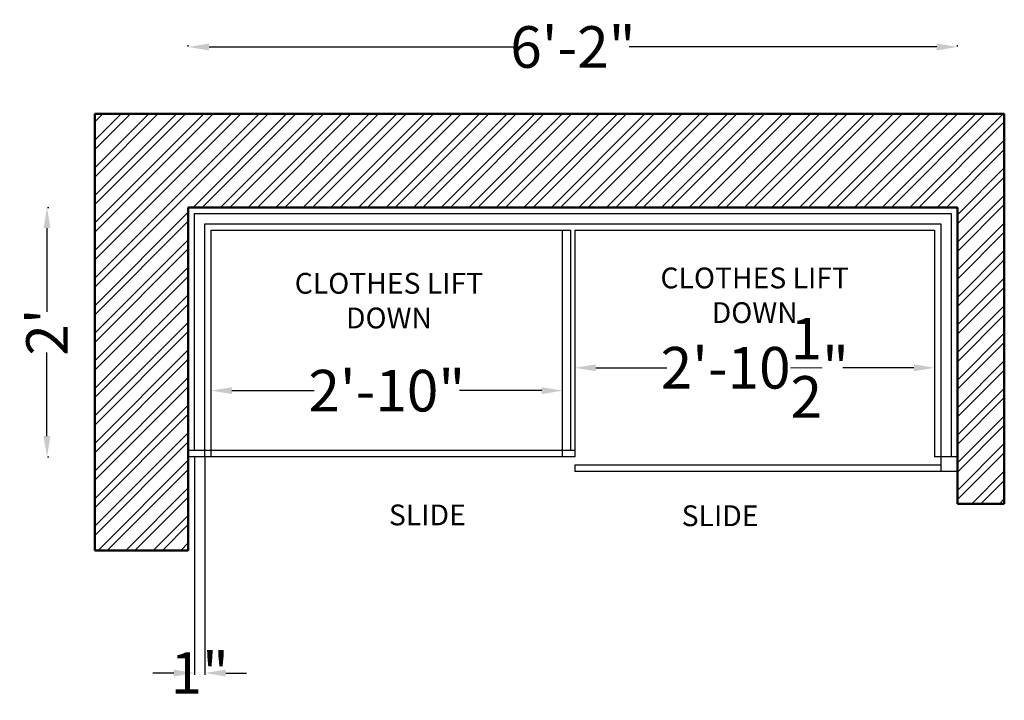
# Model space of a CAD drawing. Units: inches. Extents: x -26 to 186, y 15 to 278.
# Tile 2 of 2: x 53 to 148, y 213 to 278. Entities that reach past the tile are written whole.
import ezdxf

# ---------------------------------------------------------------- set-up
doc = ezdxf.new("R2010")
doc.units = ezdxf.units.IN
doc.header["$LTSCALE"] = 2
doc.header["$MEASUREMENT"] = 0
for name, color, linetype, lineweight in [('A-ANNO-DIMS', 2, 'Continuous', 18), ('A-ANNO-TEXT', 7, 'Continuous', 18), ('A-FURN', 3, 'Continuous', 25), ('A-WALL', 7, 'Continuous', 50), ('A-WALL-PATT', 8, 'Continuous', 18)]:
    doc.layers.add(name, color=color, linetype=linetype, lineweight=lineweight)
doc.styles.get("Standard").update_dxf_attribs({"font": 'arial.ttf'})
doc.dimstyles.get("Standard").update_dxf_attribs({"dimtxt": 4, "dimasz": 2, "dimexe": 0.18, "dimexo": 0.0625, "dimgap": 0.09, "dimtad": 0, "dimdec": 1, "dimzin": 0, "dimdsep": 46, "dimlunit": 4, "dimtxsty": 'Standard', "dimcen": 0.09, "dimadec": 0, "dimazin": 0, "dimtfac": 1, "dimtdec": 1, "dimtix": 1, "dimtofl": 0, "dimtmove": 1, "dimatfit": 2, "dimfxl": 1, "dimtolj": 1, "dimtzin": 0, "dimarcsym": 0})

# ---------------------------------------------------------------- blocks, each defined once
blk = doc.blocks.new('*D1')
at = {"layer": 'A-ANNO-DIMS', "color": 0, "lineweight": -2, "transparency": 16777216}
for p, q in [((70.275, 236.201), (70.275, 215.298)), ((71.275, 236.201), (71.275, 215.298)), ((68.275, 215.478), (66.275, 215.478)), ((73.275, 215.478), (75.275, 215.478))]:
    blk.add_line(p, q, dxfattribs=at)
at = {"layer": 'A-ANNO-DIMS', "color": 0, "transparency": 16777216}
for points in [[(68.275, 215.811), (68.275, 215.144), (70.275, 215.478)], [(73.275, 215.811), (73.275, 215.144), (71.275, 215.478)]]:
    blk.add_solid(points, dxfattribs=at)
at = {"layer": 'Defpoints', "color": 0, "transparency": 16777216}
for p in [(70.275, 236.264), (71.275, 236.264), (71.275, 215.478)]:
    blk.add_point(p, dxfattribs=at)
at = {"layer": 'A-ANNO-DIMS', "color": 0, "transparency": 16777216, "insert": (70.775, 215.478), "char_height": 4, "attachment_point": 5}
blk.add_mtext('\\A1;1"', dxfattribs=at)
blk = doc.blocks.new('*D2')
at = {"layer": 'A-ANNO-DIMS', "color": 0, "lineweight": -2, "transparency": 16777216}
for p, q in [((69.675, 275.749), (69.675, 275.867)), ((71.675, 275.687), (101.258, 275.687)), ((141.675, 275.687), (112.093, 275.687)), ((143.675, 275.749), (143.675, 275.867))]:
    blk.add_line(p, q, dxfattribs=at)
at = {"layer": 'A-ANNO-DIMS', "color": 0, "transparency": 16777216}
for points in [[(71.675, 276.02), (71.675, 275.353), (69.675, 275.687)], [(141.675, 276.02), (141.675, 275.353), (143.675, 275.687)]]:
    blk.add_solid(points, dxfattribs=at)
at = {"layer": 'Defpoints', "color": 0, "transparency": 16777216}
for p in [(69.675, 275.687), (143.675, 275.687), (143.675, 275.687)]:
    blk.add_point(p, dxfattribs=at)
at = {"layer": 'A-ANNO-DIMS', "color": 0, "transparency": 16777216, "insert": (106.675, 275.687), "char_height": 4, "attachment_point": 5}
blk.add_mtext('\\A1;6\'-2"', dxfattribs=at)
blk = doc.blocks.new('*D3')
at = {"layer": 'A-ANNO-DIMS', "color": 0, "lineweight": -2, "transparency": 16777216}
for p, q in [((71.875, 236.926), (71.875, 242.813)), ((73.875, 242.633), (81.781, 242.633)), ((103.675, 242.633), (95.77, 242.633)), ((105.675, 236.926), (105.675, 242.813))]:
    blk.add_line(p, q, dxfattribs=at)
at = {"layer": 'A-ANNO-DIMS', "color": 0, "transparency": 16777216}
for points in [[(73.875, 242.967), (73.875, 242.3), (71.875, 242.633)], [(103.675, 242.967), (103.675, 242.3), (105.675, 242.633)]]:
    blk.add_solid(points, dxfattribs=at)
at = {"layer": 'Defpoints', "color": 0, "transparency": 16777216}
for p in [(105.675, 242.633), (71.875, 236.864), (105.675, 236.864)]:
    blk.add_point(p, dxfattribs=at)
at = {"layer": 'A-ANNO-DIMS', "color": 0, "transparency": 16777216, "insert": (88.775, 242.633), "char_height": 4, "attachment_point": 5}
blk.add_mtext('\\A1;2\'-10"', dxfattribs=at)
blk = doc.blocks.new('*D4')
at = {"layer": 'A-ANNO-DIMS', "color": 0, "lineweight": -2, "transparency": 16777216}
for p, q in [((106.875, 258.001), (106.875, 244.655)), ((141.475, 258.001), (141.475, 244.655)), ((108.875, 244.835), (115.723, 244.835)), ((139.475, 244.835), (132.628, 244.835))]:
    blk.add_line(p, q, dxfattribs=at)
at = {"layer": 'A-ANNO-DIMS', "color": 0, "transparency": 16777216}
for points in [[(108.875, 245.168), (108.875, 244.502), (106.875, 244.835)], [(139.475, 245.168), (139.475, 244.502), (141.475, 244.835)]]:
    blk.add_solid(points, dxfattribs=at)
at = {"layer": 'Defpoints', "color": 0, "transparency": 16777216}
for p in [(106.875, 258.064), (141.475, 258.064), (141.475, 244.835)]:
    blk.add_point(p, dxfattribs=at)
at = {"layer": 'A-ANNO-DIMS', "color": 0, "transparency": 16777216, "insert": (124.175, 244.835), "char_height": 4, "attachment_point": 5}
blk.add_mtext('\\A1;2\'-10{\\H1x;\\S1/2;}"', dxfattribs=at)
blk = doc.blocks.new('*D5')
at = {"layer": 'A-ANNO-DIMS', "color": 0, "lineweight": -2, "transparency": 16777216}
for p, q in [((56.143, 260.264), (56.26, 260.264)), ((56.08, 258.264), (56.08, 250.228)), ((56.08, 238.264), (56.08, 246.299)), ((56.143, 236.264), (56.26, 236.264))]:
    blk.add_line(p, q, dxfattribs=at)
at = {"layer": 'A-ANNO-DIMS', "color": 0, "transparency": 16777216}
for points in [[(55.747, 258.264), (56.414, 258.264), (56.08, 260.264)], [(55.747, 238.264), (56.414, 238.264), (56.08, 236.264)]]:
    blk.add_solid(points, dxfattribs=at)
at = {"layer": 'Defpoints', "color": 0, "transparency": 16777216}
for p in [(56.08, 260.264), (56.08, 236.264), (56.08, 236.264)]:
    blk.add_point(p, dxfattribs=at)
at = {"layer": 'A-ANNO-DIMS', "color": 0, "transparency": 16777216, "insert": (56.08, 248.264), "char_height": 4, "attachment_point": 5, "rotation": 90}
blk.add_mtext("\\A1;2'", dxfattribs=at)

msp = doc.modelspace()

# ---------------------------------------------------------------- hatches: boundary and pattern name
at = {"layer": 'A-WALL-PATT'}
h = msp.add_hatch(dxfattribs=at)
h.set_pattern_fill('ANSI32', color=256, scale=5)
h.set_pattern_definition([(45, (-873.9852, -458.4655), (-1.3258252, 1.3258252), []), (45, (-873.1014, -458.4655), (-1.3258252, 1.3258252), [])])
h.paths.add_polyline_path([(60.675, 227.264), (69.675, 227.264), (69.675, 260.264), (143.675, 260.264), (143.675, 231.764), (148.175, 231.764), (148.175, 269.264), (60.675, 269.264)])

# ---------------------------------------------------------------- linework, layer by layer
at = {"layer": 'A-FURN'}
for p, q in [((71.275, 258.664), (142.075, 258.664)), ((71.875, 258.064), (106.475, 258.064)), ((106.875, 258.064), (141.475, 258.064)), ((106.875, 236.864), (69.675, 236.864)), ((106.875, 236.264), (69.675, 236.264)), ((143.675, 236.264), (141.475, 236.264)), ((142.075, 235.464), (106.875, 235.464)), ((143.675, 234.864), (106.875, 234.864))]:
    msp.add_line(p, q, dxfattribs=at)
for points in [[(70.275, 236.864), (70.275, 259.664), (143.075, 259.664), (143.075, 236.264)], [(71.275, 236.264), (71.275, 258.664)], [(142.075, 258.664), (142.075, 234.864)], [(71.875, 236.264), (71.875, 258.064)], [(105.675, 236.264), (105.675, 258.064)], [(106.475, 236.864), (106.475, 258.064)], [(106.875, 258.064), (106.875, 236.264)], [(141.475, 258.064), (141.475, 236.264)], [(106.875, 235.464), (106.875, 234.864)]]:
    msp.add_lwpolyline(points, dxfattribs=at)
at = {"layer": 'A-WALL'}
for p, q in [((60.675, 269.264), (148.175, 269.264)), ((60.675, 227.264), (60.675, 269.264)), ((148.175, 269.264), (148.175, 231.764)), ((69.675, 260.264), (143.675, 260.264)), ((69.675, 227.264), (69.675, 260.264)), ((143.675, 260.264), (143.675, 231.764)), ((148.175, 231.764), (143.675, 231.764)), ((69.675, 227.264), (60.675, 227.264))]:
    msp.add_line(p, q, dxfattribs=at)

# ---------------------------------------------------------------- texts
at = {"layer": 'A-ANNO-TEXT', "char_height": 2, "attachment_point": 1}
for s, width, insert in [('\\pxqc;CLOTHES LIFT\\PDOWN', 43.47644, (67.242, 253.956)), ('\\pxqc;CLOTHES LIFT\\PDOWN', 43.47644, (102.426, 254.472)), ('\\pxqc;SLIDE', 20.84453, (82.248, 231.683)), ('\\pxqc;SLIDE', 20.84453, (110.412, 231.604))]:
    msp.add_mtext_dynamic_manual_height_columns(s, width=width, gutter_width=10, heights=[0], dxfattribs=dict(at, insert=insert))

# ---------------------------------------------------------------- dimensions: what is measured, and where the dimension line sits
at = {"layer": 'A-ANNO-DIMS'}
for base, p1, p2, picture, middle in [((143.675, 275.687), (69.675, 275.687), (143.675, 275.687), '*D2', (106.675, 275.687)), ((141.475, 244.835), (106.875, 258.064), (141.475, 258.064), '*D4', (124.175, 244.835)), ((105.675, 242.633), (71.875, 236.864), (105.675, 236.864), '*D3', (88.775, 242.633)), ((71.275, 215.478), (70.275, 236.264), (71.275, 236.264), '*D1', (70.775, 215.478))]:
    dim = msp.add_linear_dim(base=base, p1=p1, p2=p2, dimstyle='Standard', override={"dimclrd": 0, "dimclre": 0, "dimclrt": 0}, dxfattribs=at)
    dim.commit()
    dim.dimension.update_dxf_attribs({"geometry": picture, "text_midpoint": middle})
dim = msp.add_linear_dim(base=(56.08, 236.264), p1=(56.08, 260.264), p2=(56.08, 236.264), angle=90, dimstyle='Standard', override={"dimclrd": 0, "dimclre": 0, "dimclrt": 0}, dxfattribs=at)
dim.commit()
dim.dimension.update_dxf_attribs({"geometry": '*D5', "text_midpoint": (56.08, 248.264)})

doc.saveas('drawing.dxf')
